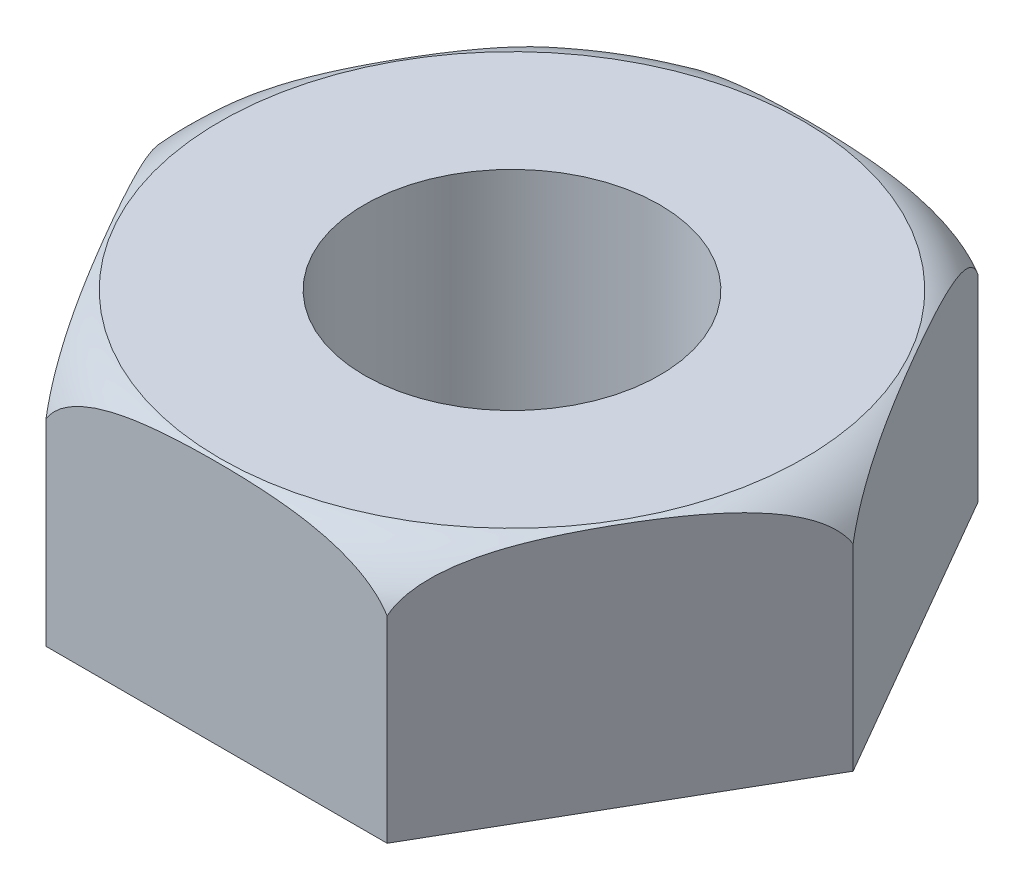
from build123d import *

# Parameters (mm, degrees)
HEX_PROFILE_SKETCH_R = 6
HEX_NUT_BODY_DEPTH   = 5


with BuildPart() as part:
    # Hex Profile Sketch → Hex Nut Body (new, symmetric)
    with BuildSketch(Plane(origin=(0, 0, 0), x_dir=(1, 0, 0), z_dir=(0, 1, 0))):
        Polygon((13.856406461, 0), (6.92820323, 12), (-6.92820323, 12), (-13.856406461, 0), (-6.92820323, -12), (6.92820323, -12), align=None)
        with Locations(Location((0, 0, 0), (0, 0, 270))):
            Circle(HEX_PROFILE_SKETCH_R, mode=Mode.SUBTRACT)
    extrude(amount=HEX_NUT_BODY_DEPTH, both=True)

    # Corner Chamfer Profile Sketch → Hex Corner Chamfer (revolve, cut)
    with BuildSketch(Plane.XY, mode=Mode.PRIVATE) as hex_corner_chamfer_sk:
        with BuildLine():
            Line((11.856406461, 5), (13.856406461, 5))
            Line((13.856406461, 5), (13.856406461, 3))
            ThreePointArc((13.856406461, 3), (13.106898111, 4.25049165), (11.856406461, 5))
        make_face()
    revolve(hex_corner_chamfer_sk.sketch.rotate(Axis((0, -7.51909737, 0), (0, 1, 0)), 90), axis=Axis((0, -7.51909737, 0), (0, 1, 0)), mode=Mode.SUBTRACT)


solid = part.part
